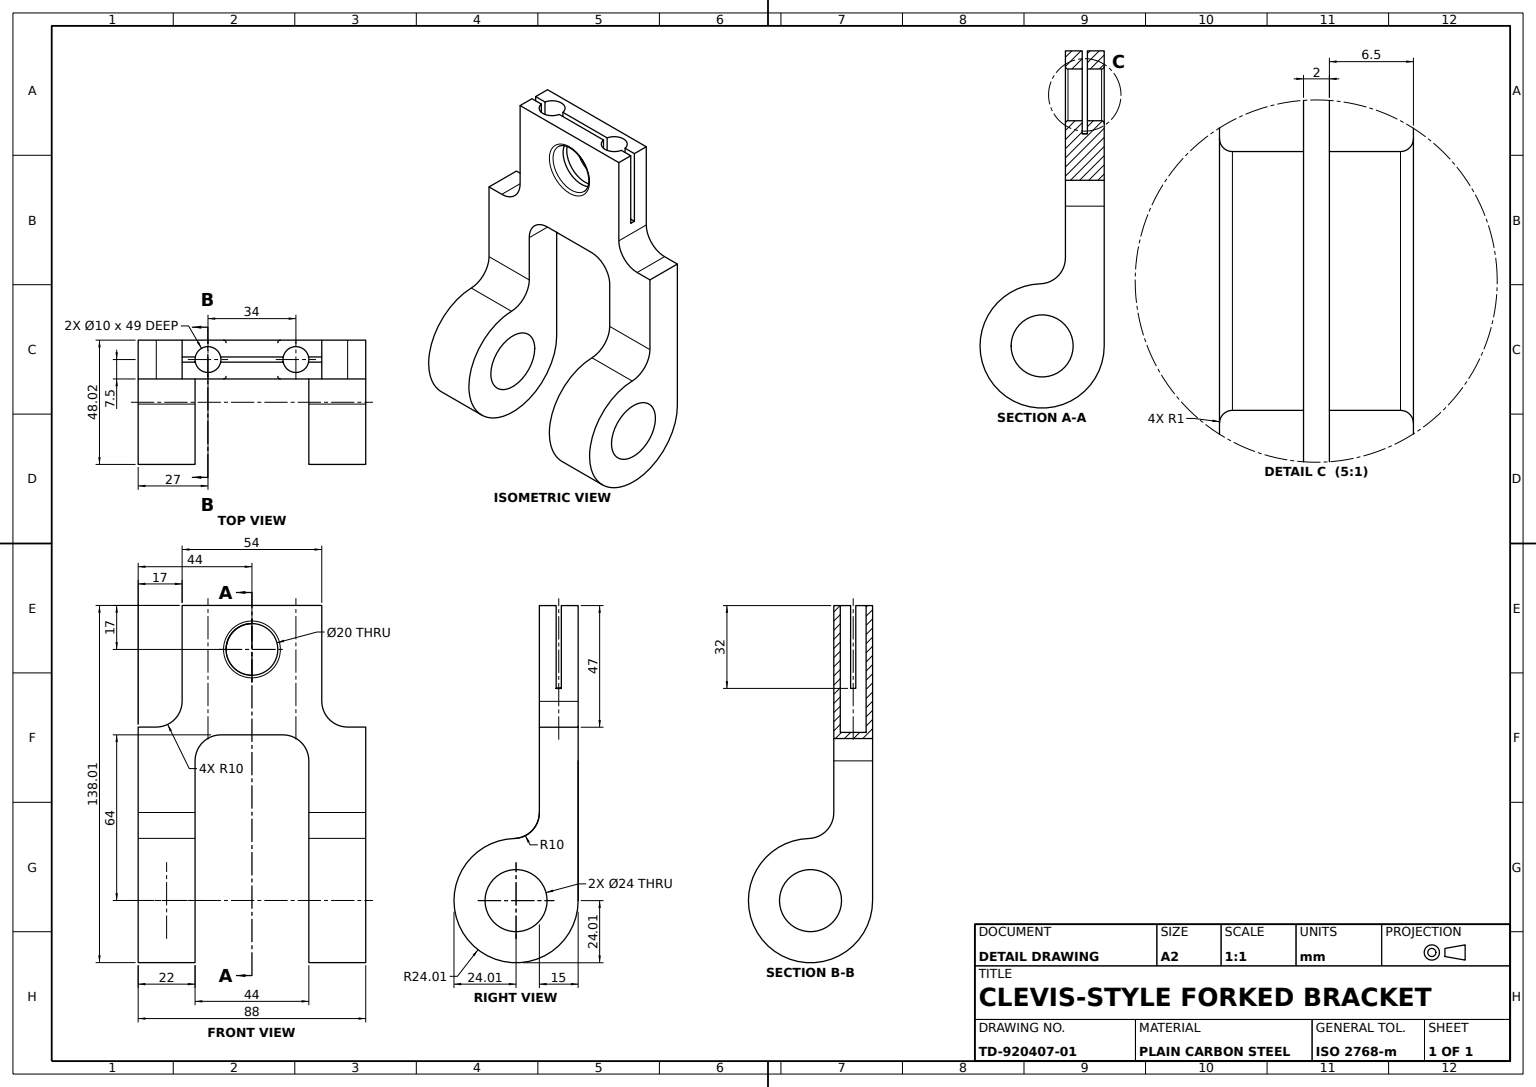
SolidWorks part; units mm, degrees
material "Plain Carbon Steel"
ref_plane "Front Plane" through (0, 0, 0) normal (0, 0, 1) x (1, 0, 0)
ref_plane "Top Plane" through (0, 0, 0) normal (0, 1, 0) x (1, 0, 0)
ref_plane "Right Plane" through (0, 0, 0) normal (1, 0, 0) x (0, 0, -1)
sketch "Lug Barrel Sketch" plane through (0, 0, 0) normal (1, 0, 0) x (0, 0, -1)
  circle A0 centre (0, 0) radius 12
  circle A1 centre (0, 0) radius 24.01
  dimension "D1" = 24.01
  dimension "D2" = 24
extrude "Roller Lug Barrel" add sketch "Lug Barrel Sketch" along normal mid plane 88
sketch "Mounting Plate Sketch" plane through (0, 0, 0) normal (1, 0, 0) x (0, 0, -1)
  line L0 (24.01, 0) -> (24.01, 114)
  line L1 (24.01, 114) -> (9.01, 114)
  line L2 (9.01, 114) -> (9.01, 22.2553)
  circle A0 centre (0, 0) radius 24.01 construction
  arc A1 (24.01, 0) -> (9.01, 22.2553) centre (0, 0) ccw
  dimension "D1" = 15
  dimension "D2" = 114
extrude "Mounting Plate" add sketch "Mounting Plate Sketch" along normal mid plane 88
fillet "Plate to Barrel Fillet R10" radius 10 1 edges at (0, 22.2553, -9.01)
sketch "Plate Shoulder Cut Sketch" plane through (0, 0, 0) normal (0, 0, 1) x (1, 0, 0)
  line L0 (-44, -24.01) -> (44, -24.01) construction
  line L1 (-22, 64) -> (22, 64)
  line L2 (-22, 64) -> (-22, -24.01)
  line L3 (-22, -24.01) -> (22, -24.01)
  line L4 (22, 64) -> (22, -24.01)
  line L5 (44, 114) -> (44, 33.9956) construction
  point P6 (0, -24.01)
  dimension "D1" = 64
  dimension "D2" = 22
extrude "Plate Shoulder Cut" cut sketch "Plate Shoulder Cut Sketch" against normal through all both and the other way through all
sketch "Lug Gap Sketch" plane through (0, 0, 0) normal (0, 0, 1) x (1, 0, 0)
  line L0 (44, 114) -> (-44, 114) construction
  line L2 (-27, 114) -> (-27, 67)
  line L4 (27, 114) -> (27, 67)
  line L5 (44, 114) -> (44, 33.9956) construction
  line L6 (-44, 114) -> (-27, 114)
  line L7 (-44, 114) -> (-44, 67)
  line L8 (-44, 67) -> (-27, 67)
  line L9 (44, 114) -> (44, 67)
  line L10 (27, 114) -> (44, 114)
  line L11 (27, 67) -> (44, 67)
  line L12 (0, 0) -> (0, 114) construction
  dimension "D1" = 47
  dimension "D2" = 54
extrude "Lug Gap Cut" cut sketch "Lug Gap Sketch" against normal through all both and the other way through all
fillet "Lug Gap Fillet R10" radius 10 4 edges at (22, 64, -16.51) (-22, 64, -16.51) (-27, 67, -16.51) (27, 67, -16.51)
sketch "Clamp Slit Sketch" plane through (0, 0, 0) normal (1, 0, 0) x (0, 0, -1)
  line L0 (24.01, 114) -> (24.01, 77) construction
  line L1 (15.51, 114) -> (17.51, 114)
  line L2 (15.51, 114) -> (15.51, 82)
  line L3 (15.51, 82) -> (17.51, 82)
  line L4 (17.51, 114) -> (17.51, 82)
  line L5 (24.01, 114) -> (9.01, 114) construction
  dimension "D1" = 6.5
  dimension "D2" = 2
  dimension "D3" = 32
extrude "Clamp Slit 2mm" cut sketch "Clamp Slit Sketch" against normal through all both and the other way through all
sketch "Plate Hole Sketch" plane through (0, 0, -9.01) normal (0, 0, 1) x (1, 0, 0)
  line L0 (27, 114) -> (-27, 114) construction
  circle A0 centre (0, 97) radius 10
  dimension "D1" = 20
  dimension "D2" = 17
extrude "Plate Hole Ø20" cut sketch "Plate Hole Sketch" against normal through all both and the other way through all
fillet "Plate Hole Edge Fillet R1" radius 1 2 edges at (0, 107, -9.01) (10, 97, -24.01)
sketch "Clamp Screw Sketch" plane through (0, 114, 0) normal (0, 1, 0) x (1, 0, 0)
  line L0 (-27, 16.51) -> (27, 16.51) construction
  line L1 (-27, 15.51) -> (-27, 17.51) construction
  line L2 (27, 17.51) -> (27, 15.51) construction
  line L5 (-10, 15.51) -> (-10, 10.01) construction
  line L6 (10, 10.01) -> (10, 15.51) construction
  circle A0 centre (-17, 16.51) radius 5
  circle A1 centre (17, 16.51) radius 5
  dimension "D3" = 10
  dimension "D1" = 7
  dimension "D2" = 7
extrude "Clamp Screw Cut" cut sketch "Clamp Screw Sketch" against normal blind 49 contours A0 | A1
